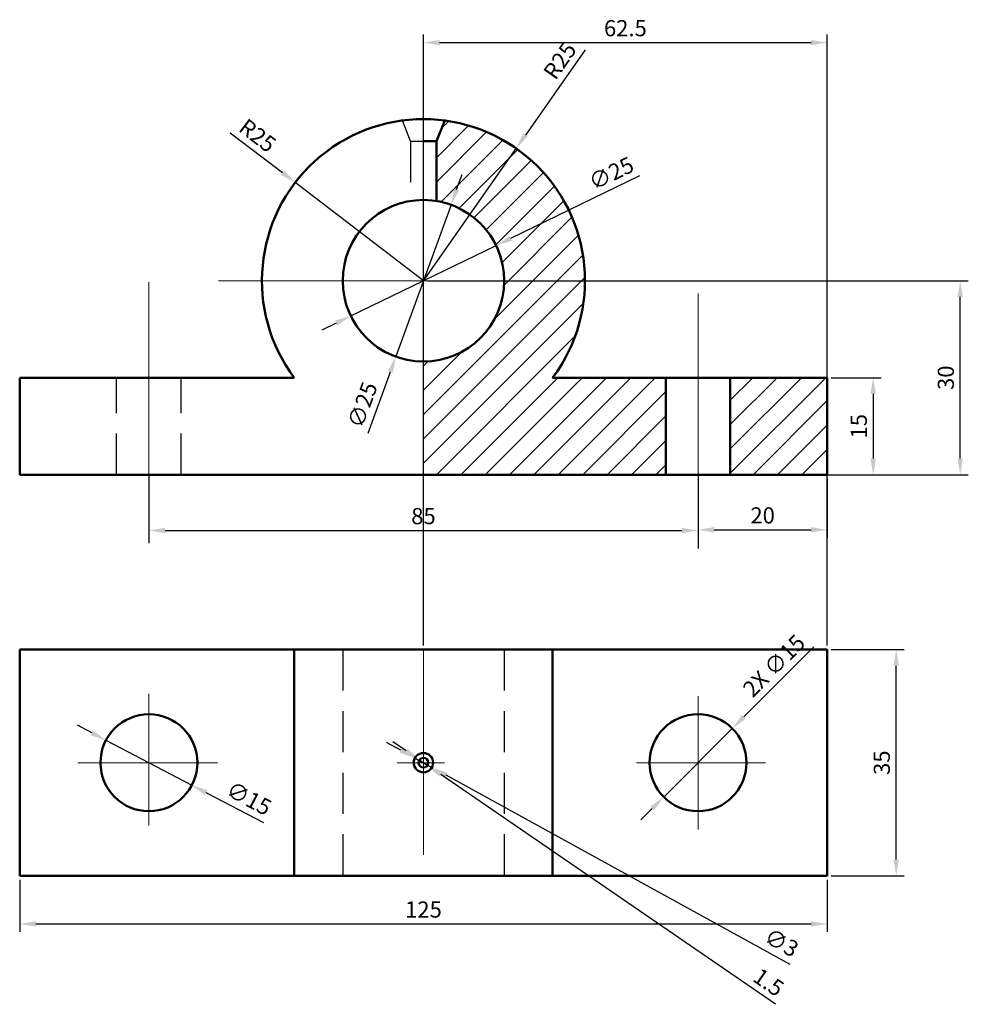
# Model space of a CAD drawing. Units: millimetres. Extents: x 2282 to 2428, y 1095 to 1247.
import ezdxf

# ---------------------------------------------------------------- set-up
doc = ezdxf.new("R2010")
doc.units = ezdxf.units.MM
doc.linetypes.add('CENTER', pattern=[50.8, 31.75, -6.35, 6.35, -6.35])
doc.linetypes.add('HIDDEN', pattern=[9.525, 6.35, -3.175])
for name, color, linetype, lineweight in [('M-CNTR', 1, 'CENTER', 18), ('M-DIMS', 2, 'Continuous', 25), ('M-HATC', 8, 'Continuous', 18), ('M-HIDN', 3, 'HIDDEN', 25), ('M-OUTL', 7, 'Continuous', 50)]:
    doc.layers.add(name, color=color, linetype=linetype, lineweight=lineweight)
doc.styles.get("Standard").update_dxf_attribs({"font": 'arial.ttf'})
doc.dimstyles.new('ISO-25', dxfattribs={"dimtxt": 2.5, "dimasz": 2.5, "dimexe": 1.25, "dimexo": 0.625, "dimtad": 1, "dimtxsty": 'Standard', "dimcen": 2.5, "dimadec": 0, "dimazin": 0, "dimtfac": 1, "dimtmove": 0, "dimatfit": 3, "dimfxl": 1, "dimarcsym": 0})

# ---------------------------------------------------------------- blocks, each defined once
blk = doc.blocks.new('*D1')
at = {"layer": 'Defpoints', "color": 0, "lineweight": -3, "transparency": 16777216}
for p in [(2324.31, 1222.15), (2344.16, 1206.94)]:
    blk.add_point(p, dxfattribs=at)
at = {"layer": 'M-DIMS', "color": 0, "lineweight": -2, "transparency": 16777216}
for p, q in [((2314.26, 1229.84), (2322.32, 1223.67)), ((2344.16, 1206.94), (2324.31, 1222.15))]:
    blk.add_line(p, q, dxfattribs=at)
at = {"layer": 'M-DIMS', "color": 0, "lineweight": -3, "transparency": 16777216}
blk.add_solid([(2322.58, 1224), (2322.07, 1223.33), (2324.31, 1222.15)], dxfattribs=at)
at = {"layer": 'M-DIMS', "color": 0, "transparency": 16777216, "insert": (2318.29, 1229.15), "char_height": 2.5, "attachment_point": 5, "rotation": 322.5465}
blk.add_mtext('R25', dxfattribs=at)
blk = doc.blocks.new('*D2')
at = {"layer": 'Defpoints', "color": 0, "lineweight": -3, "transparency": 16777216}
for p in [(2355.4, 1212.39), (2332.91, 1201.49)]:
    blk.add_point(p, dxfattribs=at)
at = {"layer": 'M-DIMS', "color": 0, "lineweight": -2, "transparency": 16777216}
for p, q in [((2377.62, 1223.16), (2357.65, 1213.48)), ((2332.91, 1201.49), (2355.4, 1212.39)), ((2330.66, 1200.4), (2328.41, 1199.31))]:
    blk.add_line(p, q, dxfattribs=at)
at = {"layer": 'M-DIMS', "color": 0, "lineweight": -3, "transparency": 16777216}
for points in [[(2357.47, 1213.86), (2357.84, 1213.11), (2355.4, 1212.39)], [(2330.48, 1200.78), (2330.84, 1200.03), (2332.91, 1201.49)]]:
    blk.add_solid(points, dxfattribs=at)
at = {"layer": 'M-DIMS', "color": 0, "transparency": 16777216, "insert": (2373.36, 1223.28), "char_height": 2.5, "attachment_point": 5, "rotation": 25.8556}
blk.add_mtext('∅25', dxfattribs=at)
blk = doc.blocks.new('*D3')
at = {"layer": 'Defpoints', "color": 0, "lineweight": -3, "transparency": 16777216}
for p in [(2301.66, 1176.94), (2386.66, 1176.94), (2386.66, 1168.31)]:
    blk.add_point(p, dxfattribs=at)
at = {"layer": 'M-DIMS', "color": 0, "lineweight": -2, "transparency": 16777216}
for p, q in [((2301.66, 1176.32), (2301.66, 1167.06)), ((2386.66, 1176.32), (2386.66, 1167.06)), ((2304.16, 1168.31), (2384.16, 1168.31))]:
    blk.add_line(p, q, dxfattribs=at)
at = {"layer": 'M-DIMS', "color": 0, "lineweight": -3, "transparency": 16777216}
for points in [[(2304.16, 1168.72), (2304.16, 1167.89), (2301.66, 1168.31)], [(2384.16, 1168.72), (2384.16, 1167.89), (2386.66, 1168.31)]]:
    blk.add_solid(points, dxfattribs=at)
at = {"layer": 'M-DIMS', "color": 0, "transparency": 16777216, "insert": (2344.16, 1170.21), "char_height": 2.5, "attachment_point": 5}
blk.add_mtext('85', dxfattribs=at)
blk = doc.blocks.new('*D4')
at = {"layer": 'Defpoints', "color": 0, "lineweight": -3, "transparency": 16777216}
for p in [(2386.66, 1176.94), (2406.66, 1176.94), (2406.66, 1168.41)]:
    blk.add_point(p, dxfattribs=at)
at = {"layer": 'M-DIMS', "color": 0, "lineweight": -2, "transparency": 16777216}
for p, q in [((2386.66, 1176.32), (2386.66, 1167.16)), ((2406.66, 1176.32), (2406.66, 1167.16)), ((2389.16, 1168.41), (2404.16, 1168.41))]:
    blk.add_line(p, q, dxfattribs=at)
at = {"layer": 'M-DIMS', "color": 0, "lineweight": -3, "transparency": 16777216}
for points in [[(2389.16, 1168.83), (2389.16, 1168), (2386.66, 1168.41)], [(2404.16, 1168.83), (2404.16, 1168), (2406.66, 1168.41)]]:
    blk.add_solid(points, dxfattribs=at)
at = {"layer": 'M-DIMS', "color": 0, "transparency": 16777216, "insert": (2396.66, 1170.32), "char_height": 2.5, "attachment_point": 5}
blk.add_mtext('20', dxfattribs=at)
blk = doc.blocks.new('*D5')
at = {"layer": 'Defpoints', "color": 0, "lineweight": -3, "transparency": 16777216}
for p in [(2406.66, 1191.94), (2406.66, 1176.94), (2413.77, 1176.94)]:
    blk.add_point(p, dxfattribs=at)
at = {"layer": 'M-DIMS', "color": 0, "lineweight": -2, "transparency": 16777216}
for p, q in [((2407.28, 1191.94), (2415.02, 1191.94)), ((2413.77, 1189.44), (2413.77, 1179.44)), ((2407.28, 1176.94), (2415.02, 1176.94))]:
    blk.add_line(p, q, dxfattribs=at)
at = {"layer": 'M-DIMS', "color": 0, "lineweight": -3, "transparency": 16777216}
for points in [[(2413.35, 1189.44), (2414.19, 1189.44), (2413.77, 1191.94)], [(2413.35, 1179.44), (2414.19, 1179.44), (2413.77, 1176.94)]]:
    blk.add_solid(points, dxfattribs=at)
at = {"layer": 'M-DIMS', "color": 0, "transparency": 16777216, "insert": (2411.87, 1184.44), "char_height": 2.5, "attachment_point": 5, "rotation": 90}
blk.add_mtext('15', dxfattribs=at)
blk = doc.blocks.new('*D6')
at = {"layer": 'Defpoints', "color": 0, "lineweight": -3, "transparency": 16777216}
for p in [(2344.16, 1206.94), (2427.24, 1206.94), (2344.16, 1176.94)]:
    blk.add_point(p, dxfattribs=at)
at = {"layer": 'M-DIMS', "color": 0, "lineweight": -2, "transparency": 16777216}
for p, q in [((2344.78, 1206.94), (2428.49, 1206.94)), ((2427.24, 1179.44), (2427.24, 1204.44)), ((2344.78, 1176.94), (2428.49, 1176.94))]:
    blk.add_line(p, q, dxfattribs=at)
at = {"layer": 'M-DIMS', "color": 0, "lineweight": -3, "transparency": 16777216}
for points in [[(2426.83, 1204.44), (2427.66, 1204.44), (2427.24, 1206.94)], [(2426.83, 1179.44), (2427.66, 1179.44), (2427.24, 1176.94)]]:
    blk.add_solid(points, dxfattribs=at)
at = {"layer": 'M-DIMS', "color": 0, "transparency": 16777216, "insert": (2425.34, 1191.94), "char_height": 2.5, "attachment_point": 5, "rotation": 90}
blk.add_mtext('30', dxfattribs=at)
blk = doc.blocks.new('*D7')
at = {"layer": 'Defpoints', "color": 0, "lineweight": -3, "transparency": 16777216}
for p in [(2406.66, 1149.89), (2417.33, 1149.89), (2406.66, 1114.89)]:
    blk.add_point(p, dxfattribs=at)
at = {"layer": 'M-DIMS', "color": 0, "lineweight": -2, "transparency": 16777216}
for p, q in [((2407.28, 1149.89), (2418.58, 1149.89)), ((2417.33, 1117.39), (2417.33, 1147.39)), ((2407.28, 1114.89), (2418.58, 1114.89))]:
    blk.add_line(p, q, dxfattribs=at)
at = {"layer": 'M-DIMS', "color": 0, "lineweight": -3, "transparency": 16777216}
for points in [[(2416.92, 1147.39), (2417.75, 1147.39), (2417.33, 1149.89)], [(2416.92, 1117.39), (2417.75, 1117.39), (2417.33, 1114.89)]]:
    blk.add_solid(points, dxfattribs=at)
at = {"layer": 'M-DIMS', "color": 0, "transparency": 16777216, "insert": (2415.43, 1132.39), "char_height": 2.5, "attachment_point": 5, "rotation": 90}
blk.add_mtext('35', dxfattribs=at)
blk = doc.blocks.new('*D8')
at = {"layer": 'Defpoints', "color": 0, "lineweight": -3, "transparency": 16777216}
for p in [(2295.01, 1135.86), (2308.3, 1128.91)]:
    blk.add_point(p, dxfattribs=at)
at = {"layer": 'M-DIMS', "color": 0, "lineweight": -2, "transparency": 16777216}
for p, q in [((2292.8, 1137.02), (2290.58, 1138.18)), ((2295.01, 1135.86), (2308.3, 1128.91)), ((2319.44, 1123.08), (2310.52, 1127.75))]:
    blk.add_line(p, q, dxfattribs=at)
at = {"layer": 'M-DIMS', "color": 0, "lineweight": -3, "transparency": 16777216}
for points in [[(2292.99, 1137.39), (2292.6, 1136.65), (2295.01, 1135.86)], [(2310.71, 1128.12), (2310.32, 1127.38), (2308.3, 1128.91)]]:
    blk.add_solid(points, dxfattribs=at)
at = {"layer": 'M-DIMS', "color": 0, "transparency": 16777216, "insert": (2317, 1126.58), "char_height": 2.5, "attachment_point": 5, "rotation": 332.3709}
blk.add_mtext('∅15', dxfattribs=at)
blk = doc.blocks.new('*D9')
at = {"layer": 'Defpoints', "color": 0, "lineweight": -3, "transparency": 16777216}
for p in [(2342.84, 1133.11), (2345.47, 1131.66)]:
    blk.add_point(p, dxfattribs=at)
at = {"layer": 'M-DIMS', "color": 0, "lineweight": -2, "transparency": 16777216}
for p, q in [((2340.65, 1134.31), (2338.46, 1135.52)), ((2342.84, 1133.11), (2345.47, 1131.66)), ((2400.94, 1101.19), (2347.66, 1130.46))]:
    blk.add_line(p, q, dxfattribs=at)
at = {"layer": 'M-DIMS', "color": 0, "lineweight": -3, "transparency": 16777216}
for points in [[(2340.85, 1134.68), (2340.45, 1133.95), (2342.84, 1133.11)], [(2347.86, 1130.83), (2347.46, 1130.09), (2345.47, 1131.66)]]:
    blk.add_solid(points, dxfattribs=at)
at = {"layer": 'M-DIMS', "color": 0, "transparency": 16777216, "insert": (2399.43, 1104.27), "char_height": 2.5, "attachment_point": 5, "rotation": 331.2143}
blk.add_mtext('∅3', dxfattribs=at)
blk = doc.blocks.new('*D10')
at = {"layer": 'Defpoints', "color": 0, "lineweight": -3, "transparency": 16777216}
for p in [(2343.54, 1132.81), (2344.77, 1131.96)]:
    blk.add_point(p, dxfattribs=at)
at = {"layer": 'M-DIMS', "color": 0, "lineweight": -2, "transparency": 16777216}
for p, q in [((2341.48, 1134.22), (2339.41, 1135.64)), ((2343.54, 1132.81), (2344.77, 1131.96)), ((2398.63, 1095.01), (2346.84, 1130.55))]:
    blk.add_line(p, q, dxfattribs=at)
at = {"layer": 'M-DIMS', "color": 0, "lineweight": -3, "transparency": 16777216}
for points in [[(2341.71, 1134.57), (2341.24, 1133.88), (2343.54, 1132.81)], [(2347.07, 1130.89), (2346.6, 1130.2), (2344.77, 1131.96)]]:
    blk.add_solid(points, dxfattribs=at)
at = {"layer": 'M-DIMS', "color": 0, "transparency": 16777216, "insert": (2397.4, 1098.16), "char_height": 2.5, "attachment_point": 5, "rotation": 325.5459}
blk.add_mtext('1.5', dxfattribs=at)
blk = doc.blocks.new('MOUNT-HOLE-D15')
blk.add_circle((0, 0), 7.5)
blk = doc.blocks.new('*D12')
at = {"layer": 'Defpoints', "color": 0, "lineweight": -3, "transparency": 16777216}
for p in [(2281.66, 1114.89), (2406.66, 1114.89), (2406.66, 1107.45)]:
    blk.add_point(p, dxfattribs=at)
at = {"layer": 'M-DIMS', "color": 0, "lineweight": -2, "transparency": 16777216}
for p, q in [((2281.66, 1114.26), (2281.66, 1106.2)), ((2406.66, 1114.26), (2406.66, 1106.2)), ((2284.16, 1107.45), (2404.16, 1107.45))]:
    blk.add_line(p, q, dxfattribs=at)
at = {"layer": 'M-DIMS', "color": 0, "lineweight": -3, "transparency": 16777216}
for points in [[(2284.16, 1107.86), (2284.16, 1107.03), (2281.66, 1107.45)], [(2404.16, 1107.86), (2404.16, 1107.03), (2406.66, 1107.45)]]:
    blk.add_solid(points, dxfattribs=at)
at = {"layer": 'M-DIMS', "color": 0, "transparency": 16777216, "insert": (2344.16, 1109.35), "char_height": 2.5, "attachment_point": 5}
blk.add_mtext('125', dxfattribs=at)
blk = doc.blocks.new('*D13')
at = {"layer": 'Defpoints', "color": 0, "lineweight": -3, "transparency": 16777216}
for p in [(2406.66, 1243.79), (2344.16, 1149.89), (2406.66, 1149.89)]:
    blk.add_point(p, dxfattribs=at)
at = {"layer": 'M-DIMS', "color": 0, "lineweight": -2, "transparency": 16777216}
for p, q in [((2344.16, 1150.51), (2344.16, 1245.04)), ((2406.66, 1150.51), (2406.66, 1245.04)), ((2346.66, 1243.79), (2404.16, 1243.79))]:
    blk.add_line(p, q, dxfattribs=at)
at = {"layer": 'M-DIMS', "color": 0, "lineweight": -3, "transparency": 16777216}
for points in [[(2346.66, 1244.2), (2346.66, 1243.37), (2344.16, 1243.79)], [(2404.16, 1244.2), (2404.16, 1243.37), (2406.66, 1243.79)]]:
    blk.add_solid(points, dxfattribs=at)
at = {"layer": 'M-DIMS', "color": 0, "transparency": 16777216, "insert": (2375.41, 1245.69), "char_height": 2.5, "attachment_point": 5}
blk.add_mtext('62.5', dxfattribs=at)
blk = doc.blocks.new('*D14')
at = {"layer": 'Defpoints', "color": 0, "lineweight": -3, "transparency": 16777216}
for p in [(2358.5, 1227.42), (2344.16, 1206.94)]:
    blk.add_point(p, dxfattribs=at)
at = {"layer": 'M-DIMS', "color": 0, "lineweight": -2, "transparency": 16777216}
for p, q in [((2369.18, 1242.67), (2359.93, 1229.47)), ((2344.16, 1206.94), (2358.5, 1227.42))]:
    blk.add_line(p, q, dxfattribs=at)
at = {"layer": 'M-DIMS', "color": 0, "lineweight": -3, "transparency": 16777216}
blk.add_solid([(2359.59, 1229.71), (2360.27, 1229.23), (2358.5, 1227.42)], dxfattribs=at)
at = {"layer": 'M-DIMS', "color": 0, "transparency": 16777216, "insert": (2365.54, 1240.8), "char_height": 2.5, "attachment_point": 5, "rotation": 55}
blk.add_mtext('R25', dxfattribs=at)
blk = doc.blocks.new('*D15')
at = {"layer": 'Defpoints', "color": 0, "lineweight": -3, "transparency": 16777216}
for p in [(2348.43, 1218.69), (2339.88, 1195.2)]:
    blk.add_point(p, dxfattribs=at)
at = {"layer": 'M-DIMS', "color": 0, "lineweight": -2, "transparency": 16777216}
for p, q in [((2349.29, 1221.04), (2350.14, 1223.39)), ((2348.43, 1218.69), (2339.88, 1195.2)), ((2335.58, 1183.38), (2339.03, 1192.85))]:
    blk.add_line(p, q, dxfattribs=at)
at = {"layer": 'M-DIMS', "color": 0, "lineweight": -3, "transparency": 16777216}
for points in [[(2348.89, 1221.18), (2349.68, 1220.9), (2348.43, 1218.69)], [(2338.63, 1192.99), (2339.42, 1192.7), (2339.88, 1195.2)]]:
    blk.add_solid(points, dxfattribs=at)
at = {"layer": 'M-DIMS', "color": 0, "transparency": 16777216, "insert": (2335.02, 1187.62), "char_height": 2.5, "attachment_point": 5, "rotation": 69.9998}
blk.add_mtext('∅25', dxfattribs=at)
blk = doc.blocks.new('*D16')
at = {"layer": 'Defpoints', "color": 0, "lineweight": -3, "transparency": 16777216}
for p in [(2391.96, 1137.69), (2381.35, 1127.08)]:
    blk.add_point(p, dxfattribs=at)
at = {"layer": 'M-DIMS', "color": 0, "lineweight": -2, "transparency": 16777216}
for p, q in [((2404.58, 1150.31), (2393.73, 1139.46)), ((2381.35, 1127.08), (2391.96, 1137.69)), ((2379.58, 1125.32), (2377.82, 1123.55))]:
    blk.add_line(p, q, dxfattribs=at)
at = {"layer": 'M-DIMS', "color": 0, "lineweight": -3, "transparency": 16777216}
for points in [[(2393.43, 1139.75), (2394.02, 1139.16), (2391.96, 1137.69)], [(2379.29, 1125.61), (2379.88, 1125.02), (2381.35, 1127.08)]]:
    blk.add_solid(points, dxfattribs=at)
at = {"layer": 'M-DIMS', "color": 0, "transparency": 16777216, "insert": (2398.64, 1147.16), "char_height": 2.5, "attachment_point": 5, "rotation": 44.9983}
blk.add_mtext('2X ∅15', dxfattribs=at)

msp = doc.modelspace()

# ---------------------------------------------------------------- hatches: boundary and pattern name
at = {"layer": 'M-HATC'}
h = msp.add_hatch(dxfattribs=at)
h.set_pattern_fill('ANSI31', color=256, scale=0.84)
h.paths.add_polyline_path([(2347.44, 1231.726), (2346.156, 1228.518), (2346.156, 1219.281, -0.3678942), (2356.656, 1206.942), (2369.156, 1206.942, 0.3761357)])
h.paths.add_polyline_path([(2369.156, 1206.942), (2356.656, 1206.942, -0.4142136), (2344.156, 1194.442), (2344.156, 1176.942), (2381.656, 1176.942), (2381.656, 1191.942), (2364.156, 1191.942, 0.1622777)])
h = msp.add_hatch(dxfattribs=at)
h.set_pattern_fill('ANSI31', color=256, scale=0.84)
h.paths.add_polyline_path([(2406.656, 1191.942), (2391.656, 1191.942), (2391.656, 1176.942), (2406.656, 1176.942)])

# ---------------------------------------------------------------- linework, layer by layer
at = {"layer": 'M-CNTR'}
for p, q in [((2344.156, 1206.942), (2344.156, 1236.346)), ((2301.656, 1176.942), (2301.656, 1206.732)), ((2344.156, 1206.942), (2309.141, 1206.942)), ((2344.156, 1176.942), (2344.156, 1206.942)), ((2344.156, 1206.942), (2390.582, 1206.942)), ((2386.656, 1176.942), (2386.656, 1204.956)), ((2344.156, 1149.886), (2344.156, 1114.886)), ((2301.656, 1143.047), (2301.656, 1122.663)), ((2386.656, 1142.695), (2386.656, 1122.032)), ((2290.635, 1132.386), (2312.293, 1132.386)), ((2342.656, 1132.386), (2340.078, 1132.386)), ((2342.656, 1132.386), (2347.39, 1132.386)), ((2377.138, 1132.386), (2397.124, 1132.386))]:
    msp.add_line(p, q, dxfattribs=at)
at = {"layer": 'M-DIMS'}
for p, q in [((2301.656, 1176.942), (2301.656, 1166.339)), ((2386.656, 1176.942), (2386.656, 1165.504))]:
    msp.add_line(p, q, dxfattribs=at)
at = {"layer": 'M-HIDN'}
for p, q in [((2342.156, 1228.518), (2340.936, 1231.734)), ((2342.156, 1228.518), (2344.156, 1228.518)), ((2342.156, 1228.518), (2342.156, 1219.281)), ((2296.656, 1176.942), (2296.656, 1191.942)), ((2306.656, 1176.942), (2306.656, 1191.942)), ((2331.656, 1149.886), (2331.656, 1114.886)), ((2356.656, 1149.886), (2356.656, 1114.886))]:
    msp.add_line(p, q, dxfattribs=at)
at = {"layer": 'M-OUTL'}
for p, q in [((2346.156, 1228.518), (2347.44, 1231.726)), ((2344.156, 1228.518), (2346.156, 1228.518)), ((2346.156, 1228.518), (2346.156, 1219.281)), ((2281.656, 1176.942), (2281.656, 1191.942)), ((2281.656, 1191.942), (2324.156, 1191.942)), ((2364.156, 1191.942), (2391.656, 1191.942)), ((2381.656, 1176.942), (2381.656, 1191.942)), ((2391.656, 1176.942), (2391.656, 1191.942)), ((2391.656, 1191.942), (2406.656, 1191.942)), ((2406.656, 1176.942), (2406.656, 1191.942)), ((2301.656, 1176.942), (2281.656, 1176.942)), ((2301.656, 1176.942), (2386.656, 1176.942)), ((2386.656, 1176.942), (2406.656, 1176.942)), ((2281.656, 1149.886), (2406.656, 1149.886)), ((2281.656, 1149.886), (2281.656, 1114.886)), ((2324.156, 1149.886), (2324.156, 1114.886)), ((2364.156, 1149.886), (2364.156, 1114.886)), ((2406.656, 1149.886), (2406.656, 1114.886)), ((2281.656, 1114.886), (2406.656, 1114.886))]:
    msp.add_line(p, q, dxfattribs=at)
for centre, radius in [((2344.156, 1206.942), 12.5), ((2344.156, 1132.386), 1.5), ((2344.156, 1132.386), 0.75)]:
    msp.add_circle(centre, radius, dxfattribs=at)
msp.add_arc((2344.156, 1206.942), 25, 323.1301, 216.8699, dxfattribs=at)

# ---------------------------------------------------------------- block references
for p in [(2301.656, 1132.386), (2386.656, 1132.386)]:
    msp.add_blockref('MOUNT-HOLE-D15', p, dxfattribs=at)

# ---------------------------------------------------------------- dimensions: what is measured, and where the dimension line sits
at = {"layer": 'M-DIMS'}
for base, p1, p2, override, picture, middle in [((2406.656, 1243.786), (2344.156, 1149.886), (2406.656, 1149.886), {"dimdec": 1, "dimlfac": 1, "dimrnd": 0, "dimzin": 0, "dimdsep": 46, "dimlunit": 2}, '*D13', (2375.406, 1245.687)), ((2386.656, 1168.305), (2301.656, 1176.942), (2386.656, 1176.942), {"dimclrd": 0, "dimclre": 0, "dimclrt": 0}, '*D3', (2344.156, 1170.207)), ((2406.656, 1168.415), (2386.656, 1176.942), (2406.656, 1176.942), {"dimclrd": 0, "dimclre": 0, "dimclrt": 0}, '*D4', (2396.656, 1170.316)), ((2406.656, 1107.446), (2281.656, 1114.886), (2406.656, 1114.886), {"dimdec": 0, "dimlfac": 1, "dimrnd": 0, "dimzin": 0, "dimdsep": 46, "dimlunit": 2}, '*D12', (2344.156, 1109.348))]:
    dim = msp.add_linear_dim(base=base, p1=p1, p2=p2, dimstyle='ISO-25', override=override, dxfattribs=at)
    dim.commit()
    dim.dimension.update_dxf_attribs({"geometry": picture, "text_midpoint": middle})
for mpoint, override, picture, middle in [((2358.495, 1227.421), {"dimdec": 0, "dimlfac": 1, "dimrnd": 0, "dimzin": 0, "dimdsep": 46, "dimlunit": 2}, '*D14', (2367.099, 1239.709)), ((2324.31, 1222.145), {"dimclrd": 0, "dimclre": 0, "dimclrt": 0}, '*D1', (2317.136, 1227.641))]:
    dim = msp.add_radius_dim(center=(2344.156, 1206.942), mpoint=mpoint, dimstyle='ISO-25', override=override, dxfattribs=at)
    dim.commit()
    dim.dimension.update_dxf_attribs({"geometry": picture, "text_midpoint": middle, "dimtype": 164})
for p1, p2, override, picture, middle in [((2332.907, 1201.491), (2355.404, 1212.394), {"dimclrd": 0, "dimclre": 0, "dimclrt": 0}, '*D2', (2374.218, 1221.511)), ((2348.431, 1218.689), (2339.88, 1195.196), {"dimdec": 0, "dimlfac": 1, "dimrnd": 0, "dimzin": 0, "dimdsep": 46, "dimlunit": 2}, '*D15', (2336.876, 1186.941)), ((2342.841, 1133.108), (2345.47, 1131.664), {"dimclrd": 0, "dimclre": 0, "dimclrt": 0}, '*D9', (2398.482, 1102.538))]:
    dim = msp.add_diameter_dim_2p(p1=p1, p2=p2, dimstyle='ISO-25', override=override, dxfattribs=at)
    dim.commit()
    dim.dimension.update_dxf_attribs({"geometry": picture, "text_midpoint": middle, "dimtype": 163})
for base, p1, p2, picture, middle in [((2427.245, 1206.942), (2344.156, 1176.942), (2344.156, 1206.942), '*D6', (2425.343, 1191.942)), ((2413.769, 1176.942), (2406.656, 1191.942), (2406.656, 1176.942), '*D5', (2411.867, 1184.442)), ((2417.333, 1149.886), (2406.656, 1114.886), (2406.656, 1149.886), '*D7', (2415.431, 1132.386))]:
    dim = msp.add_linear_dim(base=base, p1=p1, p2=p2, angle=90, dimstyle='ISO-25', override={"dimclrd": 0, "dimclre": 0, "dimclrt": 0}, dxfattribs=at)
    dim.commit()
    dim.dimension.update_dxf_attribs({"geometry": picture, "text_midpoint": middle})
for p1, p2, text, override, picture, middle in [((2381.352, 1127.083), (2391.959, 1137.689), '2X <>', {"dimdec": 0, "dimlfac": 1, "dimrnd": 0, "dimzin": 0, "dimdsep": 46, "dimlunit": 2}, '*D16', (2400.039, 1145.768)), ((2343.537, 1132.81), (2344.774, 1131.962), '1.5', {"dimclrd": 0, "dimclre": 0, "dimclrt": 0}, '*D10', (2396.328, 1096.591))]:
    dim = msp.add_diameter_dim_2p(p1=p1, p2=p2, text=text, dimstyle='ISO-25', override=override, dxfattribs=at)
    dim.commit()
    dim.dimension.update_dxf_attribs({"geometry": picture, "text_midpoint": middle, "dimtype": 163})
dim = msp.add_diameter_dim_2p(p1=(2295.011, 1135.864), p2=(2308.301, 1128.908), dimstyle='ISO-25', override={"dimclrd": 0, "dimclre": 0, "dimclrt": 0}, dxfattribs=at)
dim.commit()
dim.dimension.update_dxf_attribs({"geometry": '*D8', "text_midpoint": (2316.998, 1126.581)})

doc.saveas('drawing.dxf')
